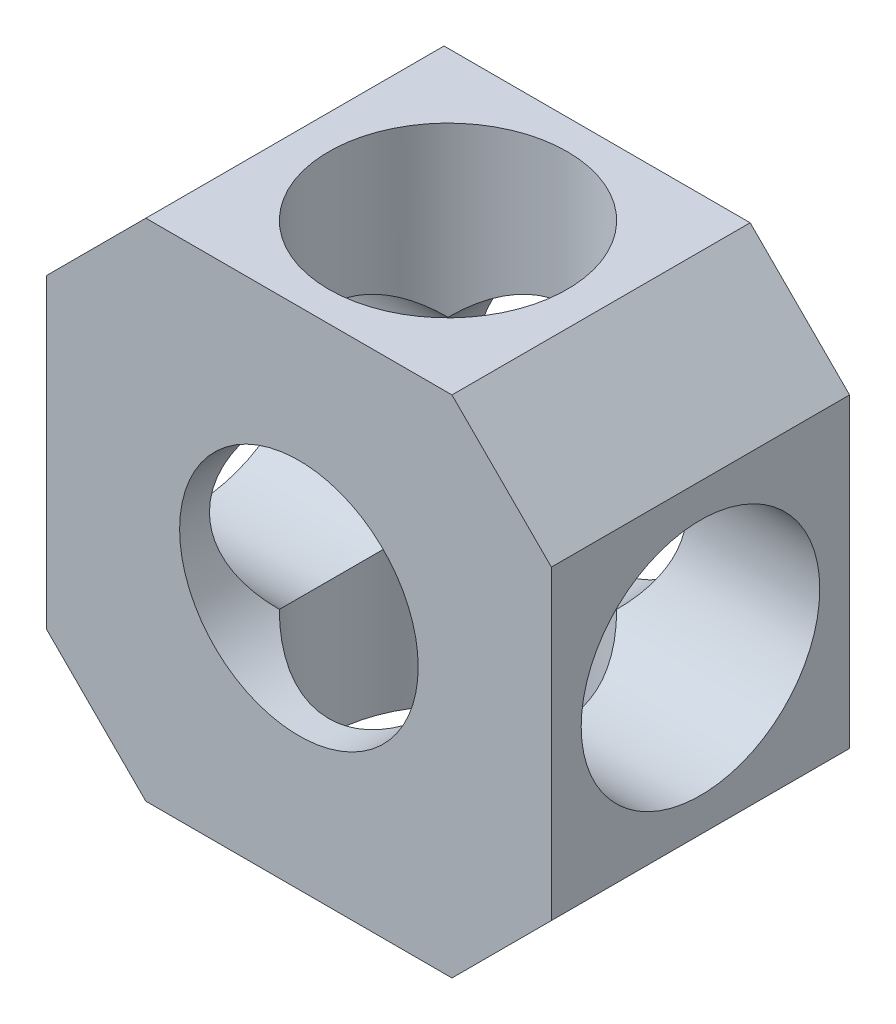
from build123d import *

# Parameters (mm, degrees)
NUT_BODY_PROFILE_W     = 25.4
NUT_BODY_PROFILE_H     = 25.4
NUT_BODY_DEPTH         = 7.5
EDGE_CHAMFERS_5MM_SIZE = 5
AXIAL_BORE_PROFILE_R   = 6
AXIAL_BORE_12_DEPTH    = 15
CROSS_BORE_A_PROFILE_R = 6
CROSS_BORE_A_12_DEPTH  = 30.37175514
CROSS_BORE_B_PROFILE_R = 6
CROSS_BORE_B_12_DEPTH  = 30.37175514


with BuildPart() as part:
    # Nut Body Profile → Nut Body (new, symmetric)
    with BuildSketch(Plane.XY):
        Rectangle(NUT_BODY_PROFILE_W, NUT_BODY_PROFILE_H)
    extrude(amount=NUT_BODY_DEPTH, both=True)

    # Edge Chamfers 5mm
    edge_chamfers_5mm_edges = [part.edges().sort_by_distance(p)[0] for p in [
        (12.7, -12.7, 0),
        (-12.7, -12.7, 0),
        (-12.7, 12.7, 0),
        (12.7, 12.7, 0),
    ]]
    chamfer(edge_chamfers_5mm_edges, length=EDGE_CHAMFERS_5MM_SIZE)

    # Axial Bore Profile → Axial Bore Ø12 (cut)
    with BuildSketch(Plane(origin=(0, 0, -7.5), x_dir=(-1, 0, 0), z_dir=(0, 0, -1))):
        Circle(AXIAL_BORE_PROFILE_R)
    extrude(amount=-AXIAL_BORE_12_DEPTH, mode=Mode.SUBTRACT)

    # Cross Bore A Profile → Cross Bore A Ø12 (cut, through all)
    with BuildSketch(Plane.ZY.offset(12.7)):
        Circle(CROSS_BORE_A_PROFILE_R)
    extrude(amount=-CROSS_BORE_A_12_DEPTH, mode=Mode.SUBTRACT)

    # Cross Bore B Profile → Cross Bore B Ø12 (cut, through all)
    with BuildSketch(Plane(origin=(0, 12.7, 0), x_dir=(1, 0, 0), z_dir=(0, 1, 0))):
        with Locations(Location((0, 0, 0), (0, 0, 270))):
            Circle(CROSS_BORE_B_PROFILE_R)
    extrude(amount=-CROSS_BORE_B_12_DEPTH, mode=Mode.SUBTRACT)


solid = part.part
